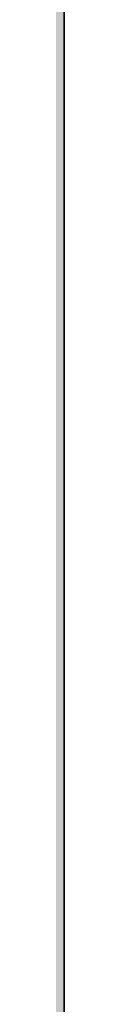
# Model space of a CAD drawing. Units: inches. Extents: x 2083 to 3317, y 1141 to 2115.
# Tile 214 of 256: x 3126.96 to 3126.96, y 1264.131 to 1265.165. Entities that reach past the tile are written whole.
import ezdxf

# ---------------------------------------------------------------- set-up
doc = ezdxf.new("R2010")
doc.units = ezdxf.units.IN
doc.layers.add('A-ANNO-DIMS', color=2, linetype='Continuous', lineweight=18)
doc.layers.add('A-WALL', color=7, linetype='Continuous', lineweight=35)
doc.layers.add('A-WALL-PATT', color=251, linetype='Continuous', lineweight=13, true_color=0x636466)
doc.styles.get("Standard").update_dxf_attribs({"font": 'arial.ttf'})
doc.dimstyles.new('ISO-25', dxfattribs={"dimtxt": 12, "dimasz": 12, "dimexe": 1.25, "dimexo": 0.625, "dimtad": 1, "dimlunit": 3, "dimtxsty": 'Standard', "dimcen": 2.5, "dimadec": 0, "dimazin": 0, "dimtfac": 1, "dimtmove": 0, "dimatfit": 3, "dimfxl": 1, "dimarcsym": 0})

# ---------------------------------------------------------------- blocks, each defined once
blk = doc.blocks.new('*D9')
at = {"layer": 'A-ANNO-DIMS', "color": 0, "lineweight": -2, "transparency": 16777216}
for p, q in [((3127.5848, 1486.7614), (3190.4031, 1486.7614)), ((3189.1531, 1474.7614), (3189.1531, 1275.2614)), ((3127.5848, 1263.2614), (3190.4031, 1263.2614))]:
    blk.add_line(p, q, dxfattribs=at)
at = {"layer": 'A-ANNO-DIMS', "color": 0, "transparency": 16777216}
for points in [[(3187.1531, 1474.7614), (3191.1531, 1474.7614), (3189.1531, 1486.7614)], [(3187.1531, 1275.2614), (3191.1531, 1275.2614), (3189.1531, 1263.2614)]]:
    blk.add_solid(points, dxfattribs=at)
at = {"layer": 'Defpoints', "color": 0, "transparency": 16777216}
for p in [(3126.9598, 1486.7614), (3126.9598, 1263.2614), (3189.1531, 1263.2614)]:
    blk.add_point(p, dxfattribs=at)
at = {"layer": 'A-ANNO-DIMS', "color": 0, "transparency": 16777216, "insert": (3182.4012, 1375.0114), "char_height": 12, "attachment_point": 5, "rotation": 90}
blk.add_mtext('18\'-7.5"', dxfattribs=at)
blk = doc.blocks.new('*D26')
at = {"layer": 'A-ANNO-DIMS', "color": 0, "lineweight": -2, "transparency": 16777216}
for p, q in [((3088.9858, 1274.9151), (3088.9858, 1270.952)), ((3111.24, 1274.9151), (3111.24, 1270.952)), ((3076.9858, 1272.202), (2840.2624, 1272.202)), ((3111.24, 1272.202), (3088.9858, 1272.202)), ((3123.24, 1272.202), (3135.24, 1272.202))]:
    blk.add_line(p, q, dxfattribs=at)
at = {"layer": 'A-ANNO-DIMS', "color": 0, "transparency": 16777216}
for points in [[(3076.9858, 1274.202), (3076.9858, 1270.202), (3088.9858, 1272.202)], [(3123.24, 1274.202), (3123.24, 1270.202), (3111.24, 1272.202)]]:
    blk.add_solid(points, dxfattribs=at)
at = {"layer": 'Defpoints', "color": 0, "transparency": 16777216}
for p in [(3088.9858, 1275.5401), (3111.24, 1275.5401), (3088.9858, 1272.202)]:
    blk.add_point(p, dxfattribs=at)
at = {"layer": 'A-ANNO-DIMS', "color": 0, "transparency": 16777216, "insert": (2952.6241, 1279.0316), "char_height": 12, "attachment_point": 5}
blk.add_mtext('NIGHTSTAND 1\'-10 1/2" TYP.', dxfattribs=at)
blk = doc.blocks.new('*D27')
at = {"layer": 'A-ANNO-DIMS', "color": 0, "lineweight": -2, "transparency": 16777216}
for p, q in [((3114.5782, 1309.7943), (3114.5782, 1321.7943)), ((3111.865, 1297.7943), (3115.8282, 1297.7943)), ((3114.5782, 1297.7943), (3114.5782, 1275.5401)), ((3111.865, 1275.5401), (3115.8282, 1275.5401)), ((3114.5782, 1263.5401), (3114.5782, 1140.9886))]:
    blk.add_line(p, q, dxfattribs=at)
at = {"layer": 'A-ANNO-DIMS', "color": 0, "transparency": 16777216}
for points in [[(3112.5782, 1309.7943), (3116.5782, 1309.7943), (3114.5782, 1297.7943)], [(3112.5782, 1263.5401), (3116.5782, 1263.5401), (3114.5782, 1275.5401)]]:
    blk.add_solid(points, dxfattribs=at)
at = {"layer": 'Defpoints', "color": 0, "transparency": 16777216}
for p in [(3111.24, 1297.7943), (3111.24, 1275.5401), (3114.5782, 1275.5401)]:
    blk.add_point(p, dxfattribs=at)
at = {"layer": 'A-ANNO-DIMS', "color": 0, "transparency": 16777216, "insert": (3107.7485, 1196.2643), "char_height": 12, "attachment_point": 5, "rotation": 90}
blk.add_mtext('1\'-10 1/2" TYP.', dxfattribs=at)

msp = doc.modelspace()

# ---------------------------------------------------------------- hatches: boundary and pattern name
at = {"layer": 'A-WALL-PATT'}
h = msp.add_hatch(color=256, dxfattribs=at)
h.dxf.hatch_style = 1
h.paths.add_polyline_path([(3126.9598, 2020.7614), (2748.9598, 2020.7614), (2604.9598, 2020.7614), (2226.9598, 2020.7614), (2226.9598, 1702.7614), (2466.9598, 1702.7614), (2466.9598, 1582.7614), (2418.9598, 1582.7614), (2418.9598, 1477.7614), (2226.9598, 1477.7614), (2226.9598, 1263.2614), (2544.9598, 1263.2614), (2544.9598, 1411.7614), (2604.9598, 1411.7614), (2685.9598, 1411.7614), (2685.9598, 1420.7614), (2604.9598, 1420.7614), (2604.9598, 1573.7614), (2604.9598, 1702.7614), (2604.9598, 2011.7614), (2748.9598, 2011.7614), (2748.9598, 1702.7614), (2862.9598, 1702.7614), (2862.9598, 1621.7614), (2871.9598, 1621.7614), (2871.9598, 1702.7614), (2883.9598, 1702.7614), (2883.9598, 1706.9395, -0.026459), (2883.9598, 1711.7614), (2757.9598, 1711.7614), (2757.9598, 1807.7614), (2787.9598, 1807.7614), (2787.9598, 1812.2614), (2757.9598, 1812.2614), (2757.9598, 2011.7614), (2877.9598, 2011.7614), (2877.9598, 1812.2614), (2847.9598, 1812.2614), (2847.9598, 1807.7614), (2889.8357, 1807.7614), (2889.8357, 1812.2614), (2882.4598, 1812.2614), (2882.4598, 2011.7614), (3117.9598, 2011.7614), (3117.9598, 1812.2614), (2937.8357, 1812.2614), (2937.8357, 1807.7614), (2995.7098, 1807.7614), (2995.7098, 1796.1177), (3000.2098, 1796.1177), (3000.2098, 1807.7614), (3117.9598, 1807.7614), (3117.9598, 1711.7614), (3000.2098, 1711.7614), (3000.2098, 1760.1177), (2998.5727, 1760.1177, -0.020711), (2995.7098, 1760.1177), (2995.7098, 1711.7614), (2931.9598, 1711.7614), (2931.9598, 1702.7614), (3126.9598, 1702.7614)])
h.paths.add_polyline_path([(2471.4598, 2011.7614), (2471.4598, 1810.0114), (2462.7169, 1810.0114), (2462.7169, 1805.5114), (2505.9598, 1805.5114), (2505.9598, 1810.0114), (2475.9598, 1810.0114), (2475.9598, 2011.7614), (2595.9598, 2011.7614), (2595.9598, 1810.0114), (2565.9598, 1810.0114), (2565.9598, 1805.5114), (2595.9598, 1805.5114), (2595.9598, 1711.7614), (2235.9598, 1711.7614), (2235.9598, 1805.5114), (2353.7098, 1805.5114), (2353.7098, 1796.0542), (2358.2098, 1796.0542), (2358.2098, 1805.5114), (2414.7169, 1805.5114), (2414.7169, 1810.0114), (2235.9598, 1810.0114), (2235.9598, 2011.7614)], flags=16)
h.paths.add_polyline_path([(2270.2047, 1994.61), (2270.2047, 1970.61), (2246.2047, 1970.61), (2246.2047, 1994.61)], flags=0)
edge = h.paths.add_edge_path(flags=0)
edge.add_ellipse((2332.0274, 1899.7982), major_axis=(-3.043, 3.043), ratio=0.168252, start_angle=-161.3322, end_angle=-156.3071, ccw=False)
edge.add_ellipse((2333.082, 1898.7435), major_axis=(-1.0546, 1.0546), ratio=0.453532, start_angle=-123.371, end_angle=-94.1591)
edge = h.paths.add_edge_path(flags=0)
edge.add_ellipse((2332.0274, 1968.8763), major_axis=(3.043, 3.043), ratio=0.168252, start_angle=18.6678, end_angle=23.6929)
edge.add_spline(control_points=[(2332.9256, 1970.6911), (2332.2268, 1970.3361), (2330.8937, 1969.6589), (2328.4131, 1970.9321), (2327.2039, 1967.7487), (2324.7096, 1969.9556), (2322.5328, 1967.0124), (2320.0128, 1971.2958), (2317.6803, 1968.1578), (2316.0405, 1967.102), (2315.4269, 1966.8096)], knot_values=[0, 0, 0, 0, 2.267059, 4.324559, 6.685584, 8.878641, 11.121502, 14.300359, 17.755284, 19.732645, 19.732645, 19.732645, 19.732645], degree=3, periodic=0)
edge.add_ellipse((2332.0274, 1968.8763), major_axis=(3.043, 3.043), ratio=0.168252, start_angle=18.6678, end_angle=23.6929, ccw=False)
edge.add_ellipse((2333.082, 1969.9309), major_axis=(1.0546, 1.0546), ratio=0.453532, start_angle=56.629, end_angle=85.8409, ccw=False)
edge = h.paths.add_edge_path(flags=0)
edge.add_spline(control_points=[(2296.4283, 1967.9879), (2293.6278, 1965.3363), (2287.7036, 1959.7271), (2299.7439, 1949.9957), (2294.5326, 1935.6685), (2290.5732, 1920.6035), (2293.3941, 1909.9737), (2296.1854, 1904.9665)], knot_values=[0.099185, 0.099185, 0.099185, 0.099185, 0.345301, 0.619822, 0.982653, 1.386093, 1.810555, 1.810555, 1.810555, 1.810555], degree=3, periodic=0)
edge.add_spline(control_points=[(2296.1854, 1904.9665), (2297.3836, 1902.6193), (2298.001, 1901.9493), (2298.553, 1901.4682)], knot_values=[0.006246, 0.006246, 0.006246, 0.006246, 0.055476, 0.055476, 0.055476, 0.055476], degree=3, periodic=0)
edge.add_spline(control_points=[(2298.553, 1901.4682), (2297.2586, 1900.9232), (2295.2253, 1900.2321), (2293.0602, 1900.6142), (2292.1014, 1900.7884), (2292.0896, 1900.7906)], knot_values=[0.312835, 0.312835, 0.312835, 0.312835, 0.40178, 0.474987, 0.475903, 0.475903, 0.475903, 0.475903], degree=3, periodic=0)
edge.add_arc((2292.7936, 1904.6641), 3.937, 215.4209, 259.6982, ccw=False)
edge.add_spline(control_points=[(2289.5853, 1902.3823), (2289.4767, 1902.5351), (2289.3685, 1902.688), (2289.2609, 1902.8412)], knot_values=[0.102872, 0.102872, 0.102872, 0.102872, 0.116896, 0.116896, 0.116896, 0.116896], degree=3, periodic=0)
edge.add_spline(control_points=[(2289.2609, 1902.8412), (2288.6866, 1902.5502), (2287.64, 1902.0199), (2285.8813, 1901.874), (2283.853, 1901.5044), (2281.72, 1899.7105), (2278.467, 1899.4929), (2276.1571, 1901.8832), (2272.259, 1899.8041), (2267.7776, 1901.8432), (2262.2439, 1900.184), (2257.4149, 1901.7821), (2254.3184, 1900.7261), (2253.1783, 1900.3373)], knot_values=[0, 0, 0, 0, 1.907977, 3.477176, 5.261074, 7.972851, 11.680248, 13.717921, 16.939592, 22.789562, 27.502503, 33.595215, 37.145618, 37.145618, 37.145618, 37.145618], degree=3, periodic=0)
edge.add_line((2253.1783, 1900.3373), (2250.2442, 1902.8412))
edge.add_line((2250.2442, 1902.8412), (2250.2442, 1965.8333))
edge.add_line((2250.2442, 1965.8333), (2253.1783, 1968.3371))
edge.add_spline(control_points=[(2253.1783, 1968.3371), (2254.3184, 1967.9483), (2257.4149, 1966.8924), (2262.2439, 1968.4904), (2267.7776, 1966.8313), (2271.5267, 1968.5372), (2273.8759, 1967.8283), (2274.2067, 1967.7276)], knot_values=[0, 0, 0, 0, 0.09018, 0.244935, 0.364644, 0.513233, 0.537855, 0.537855, 0.537855, 0.537855], degree=3, periodic=0)
edge.add_arc((2274.3529, 1963.7933), 3.937, 72.0511, 92.1279, ccw=False)
edge.add_arc((2281.2969, 1985.23), 18.5963, 252.05113, 288.56572)
edge.add_arc((2292.3167, 1956.0289), 12.6461, 71.02679, 113.77822, ccw=False)
edge = h.paths.add_edge_path(flags=0)
edge.add_spline(control_points=[(2274.8994, 1951.8562), (2275.0662, 1951.6166), (2275.2327, 1951.3766), (2275.398, 1951.1359)], knot_values=[1.409916, 1.409916, 1.409916, 1.409916, 1.43159, 1.43159, 1.43159, 1.43159], degree=3, periodic=0)
edge.add_spline(control_points=[(2275.398, 1951.1359), (2275.7921, 1950.5619), (2276.1792, 1949.9838), (2276.5455, 1949.3971)], knot_values=[1.358238, 1.358238, 1.358238, 1.358238, 1.409916, 1.409916, 1.409916, 1.409916], degree=3, periodic=0)
edge.add_line((2276.5455, 1949.3971), (2277.4373, 1947.8622))
edge.add_spline(control_points=[(2277.4373, 1947.8622), (2276.3038, 1945.6731), (2274.6397, 1942.4269), (2274.6316, 1938.0939), (2272.7991, 1930.8515), (2274.3564, 1943.897), (2275.9477, 1947.9234), (2276.5455, 1949.3971)], knot_values=[0.005632, 0.005632, 0.005632, 0.005632, 0.186014, 0.266002, 0.357087, 0.59639, 0.739732, 0.739732, 0.739732, 0.739732], degree=3, periodic=0)
edge.add_spline(control_points=[(2276.5455, 1949.3971), (2276.1792, 1949.9838), (2275.7921, 1950.5619), (2275.398, 1951.1359)], knot_values=[1.358238, 1.358238, 1.358238, 1.358238, 1.409916, 1.409916, 1.409916, 1.409916], degree=3, periodic=0)
edge.add_spline(control_points=[(2275.398, 1951.1359), (2274.9425, 1950.0805), (2274.2078, 1948.0253), (2273.9346, 1944.8515), (2272.4685, 1937.6275), (2273.4662, 1945.6965), (2274.7006, 1951.0595), (2274.8994, 1951.8562)], knot_values=[0.104364, 0.104364, 0.104364, 0.104364, 0.189636, 0.269624, 0.36071, 0.600013, 0.644622, 0.644622, 0.644622, 0.644622], degree=3, periodic=0)
h.paths.add_polyline_path([(2269.1675, 1963.1276, -0.357527), (2268.1706, 1960.9764, -0.092561), (2268.1706, 1939.4363, -0.357527), (2269.1675, 1937.2851, -0.357527), (2267.0163, 1938.282, -0.164785), (2254.6856, 1938.282, -0.357527), (2252.5344, 1937.2851, -0.357527), (2253.5313, 1939.4363, -0.092561), (2253.5313, 1960.9764, -0.357527), (2252.5344, 1963.1276, -0.357527), (2254.6856, 1962.1307, -0.164785), (2267.0163, 1962.1307, -0.357527)], flags=0)
h.paths.add_polyline_path([(2248.8741, 1967.8018), (2248.8741, 1957.0277), (2249.4578, 1957.0277), (2249.4578, 1911.6468), (2248.8741, 1911.6468), (2248.8741, 1900.8727), (2246.5119, 1900.8727, 0.197327), (2244.1497, 1902.4569), (2244.1497, 1966.2176, 0.197327), (2246.5119, 1967.8018)], flags=0)
h.paths.add_polyline_path([(2269.1675, 1931.3893, -0.357527), (2268.1706, 1929.2381, -0.092561), (2268.1706, 1907.6981, -0.357527), (2269.1675, 1905.5469, -0.357527), (2267.0163, 1906.5438, -0.164785), (2254.6856, 1906.5438, -0.357527), (2252.5344, 1905.5469, -0.357527), (2253.5313, 1907.6981, -0.092561), (2253.5313, 1929.2381, -0.357527), (2252.5344, 1931.3893, -0.357527), (2254.6856, 1930.3925, -0.164785), (2267.0163, 1930.3925, -0.357527)], flags=0)
edge = h.paths.add_edge_path(flags=0)
edge.add_spline(control_points=[(2276.1969, 1906.7237), (2276.1681, 1909.0289), (2276.114, 1913.3719), (2270.5984, 1924.925), (2273.9052, 1919.0128), (2275.9217, 1916.2621), (2275.4746, 1912.4021), (2277.2579, 1910.3806), (2276.696, 1908.225), (2276.6462, 1906.813), (2276.6178, 1906.0084)], knot_values=[0, 0, 0, 0, 8.61026, 16.221274, 18.843057, 23.804898, 27.440828, 29.356102, 31.203478, 33.650687, 33.650687, 33.650687, 33.650687], degree=3, periodic=0)
edge.add_spline(control_points=[(2276.6178, 1906.0084), (2276.6233, 1905.6241), (2276.4977, 1904.6287), (2275.4418, 1903.8547), (2274.9373, 1903.0804), (2274.8591, 1902.8412)], knot_values=[0.156488, 0.156488, 0.156488, 0.156488, 0.184398, 0.231376, 0.250598, 0.250598, 0.250598, 0.250598], degree=3, periodic=0)
edge.add_line((2274.8591, 1902.8412), (2276.506, 1902.8412))
edge.add_spline(control_points=[(2276.506, 1902.8412), (2276.7883, 1903.0849), (2277.6651, 1904.1252), (2278.2495, 1904.3407), (2277.6539, 1908.5274), (2278.1557, 1906.2278), (2278.1005, 1905.2859), (2278.8467, 1904.069), (2277.8568, 1903.4149), (2277.8742, 1902.991), (2277.9036, 1902.8412)], knot_values=[0.059574, 0.059574, 0.059574, 0.059574, 0.080753, 0.103741, 0.16972, 0.176036, 0.207137, 0.240474, 0.262341, 0.27366, 0.27366, 0.27366, 0.27366], degree=3, periodic=0)
edge.add_line((2277.9036, 1902.8412), (2280.0298, 1902.8412))
edge.add_spline(control_points=[(2280.0298, 1902.8412), (2279.8882, 1903.0884), (2279.4993, 1903.9816), (2280.1523, 1905.9393), (2278.1036, 1909.6578), (2279.7624, 1907.1853), (2280.3279, 1904.8749), (2280.4851, 1903.4896), (2281.4633, 1903.2494), (2281.7583, 1902.9365), (2281.834, 1902.8412)], knot_values=[0.013856, 0.013856, 0.013856, 0.013856, 0.034874, 0.088867, 0.107879, 0.126738, 0.158714, 0.193757, 0.217487, 0.226722, 0.226722, 0.226722, 0.226722], degree=3, periodic=0)
edge.add_spline(control_points=[(2281.834, 1902.8412), (2281.7875, 1902.8267), (2281.647, 1902.783), (2281.3955, 1902.8595), (2281.0881, 1902.9852), (2280.7207, 1903.0609), (2280.3335, 1903.0257), (2280.1248, 1902.8989), (2280.0298, 1902.8412)], knot_values=[0, 0, 0, 0, 0.14413, 0.435517, 0.749276, 1.153046, 1.548371, 1.878348, 1.878348, 1.878348, 1.878348], degree=3, periodic=0)
edge.add_line((2280.0298, 1902.8412), (2277.9036, 1902.8412))
edge.add_spline(control_points=[(2277.9036, 1902.8412), (2277.8929, 1902.7959), (2277.8654, 1902.6796), (2277.6075, 1902.6875), (2277.2741, 1902.8007), (2276.8379, 1902.6198), (2276.5838, 1902.7893), (2276.506, 1902.8412)], knot_values=[0, 0, 0, 0, 0.127189, 0.326199, 0.628009, 1.24357, 1.515331, 1.515331, 1.515331, 1.515331], degree=3, periodic=0)
edge.add_line((2276.506, 1902.8412), (2274.8591, 1902.8412))
edge.add_spline(control_points=[(2274.8591, 1902.8412), (2274.8144, 1902.8986), (2274.7251, 1903.0134), (2274.4935, 1903.119), (2274.2443, 1902.9605), (2273.9371, 1903.1849), (2273.614, 1902.9831), (2273.4083, 1902.883), (2273.3223, 1902.8412)], knot_values=[0, 0, 0, 0, 0.21843, 0.436957, 0.687977, 0.990379, 1.398396, 1.69185, 1.69185, 1.69185, 1.69185], degree=3, periodic=0)
edge.add_spline(control_points=[(2273.3223, 1902.8412), (2273.6167, 1903.4457), (2274.274, 1904.5383), (2276.0272, 1904.5737), (2276.207, 1906.5836), (2276.1969, 1906.7237)], knot_values=[0.012227, 0.012227, 0.012227, 0.012227, 0.059472, 0.106218, 0.134458, 0.134458, 0.134458, 0.134458], degree=3, periodic=0)
h.paths.add_polyline_path([(2270.7761, 1897.7898), (2270.7761, 1873.7898), (2246.7761, 1873.7898), (2246.7761, 1897.7898)], flags=0)
h.paths.add_polyline_path([(2353.7098, 1760.0051), (2353.7098, 1760.0542), (2358.2098, 1760.0542, -0.033729)], flags=0)
h.paths.add_polyline_path([(2321.8191, 1737.5292), (2341.9953, 1737.5292, -0.414214), (2343.2033, 1736.3212), (2343.2033, 1721.0206, -0.414214), (2341.9953, 1719.8127), (2321.8191, 1719.8127, -0.414214), (2320.6112, 1721.0206), (2320.6112, 1736.3212, -0.414214)], flags=0)
h.paths.add_polyline_path([(2324.235, 1736.3212), (2339.5794, 1736.3212, -0.414214), (2341.9953, 1733.9053), (2341.9953, 1725.4497, -0.414214), (2339.5794, 1723.0338), (2333.6806, 1723.0338), (2333.8453, 1722.0455, -0.870646), (2335.4254, 1721.8259, -0.767327), (2333.9227, 1721.4232), (2331.291, 1721.4232, -0.767327), (2329.7883, 1721.8259, -0.870646), (2331.3684, 1722.0455), (2331.5331, 1723.0338), (2324.235, 1723.0338, -0.414214), (2321.8191, 1725.4497), (2321.8191, 1733.9053, -0.414214)], flags=0)
h.paths.add_polyline_path([(2570.4838, 1928.6154), (2589.6838, 1928.6154), (2590.1688, 1928.6154), (2590.1688, 1904.9934), (2570.4838, 1904.9934)], flags=0)
h.paths.add_polyline_path([(2574.4473, 1927.2638, -1), (2572.8288, 1927.2638, -1)], flags=0)
h.paths.add_polyline_path([(2573.0899, 1926.9409), (2573.925, 1927.776), (2574.1477, 1927.5533), (2573.3126, 1926.7182)], flags=0)
h.paths.add_polyline_path([(2578.7791, 1919.7296, -1), (2571.5917, 1919.7296, -1)], flags=0)
h.paths.add_polyline_path([(2578.3854, 1919.7296, -1), (2571.9854, 1919.7296, -1)], flags=0)
h.paths.add_polyline_path([(2331.5958, 1729.4762, -1), (2333.618, 1729.4762, -1)], flags=0)
h.paths.add_polyline_path([(2578.0342, 1927.2638, -1), (2576.4157, 1927.2638, -1)], flags=0)
h.paths.add_polyline_path([(2576.6889, 1927.5311), (2576.9116, 1927.7538), (2577.7467, 1926.9186), (2577.524, 1926.6959)], flags=0)
h.paths.add_polyline_path([(2578.1391, 1909.8595, -1), (2572.2317, 1909.8595, -1)], flags=0)
h.paths.add_polyline_path([(2577.7454, 1909.8595, -1), (2572.6254, 1909.8595, -1)], flags=0)
h.paths.add_polyline_path([(2583.7977, 1927.2638, -1), (2582.1792, 1927.2638, -1)], flags=0)
h.paths.add_polyline_path([(2582.7186, 1927.7538), (2583.5538, 1926.9186), (2583.3311, 1926.6959), (2582.4959, 1927.5311)], flags=0)
h.paths.add_polyline_path([(2582.4959, 1927.5311), (2582.7186, 1927.7538), (2583.5538, 1926.9186), (2583.3311, 1926.6959)], flags=0)
h.paths.add_polyline_path([(2587.7391, 1920.5296, -1), (2581.8317, 1920.5296, -1)], flags=0)
h.paths.add_polyline_path([(2587.3454, 1920.5296, -1), (2582.2254, 1920.5296, -1)], flags=0)
h.paths.add_polyline_path([(2587.3846, 1927.2638, -1), (2585.7661, 1927.2638, -1)], flags=0)
h.paths.add_polyline_path([(2586.082, 1926.9802), (2586.9172, 1927.8154), (2587.1399, 1927.5927), (2586.3047, 1926.7575)], flags=0)
h.paths.add_polyline_path([(2588.3791, 1910.6595, -1), (2581.1917, 1910.6595, -1)], flags=0)
h.paths.add_polyline_path([(2587.9854, 1910.6595, -1), (2581.5854, 1910.6595, -1)], flags=0)
h.paths.add_polyline_path([(2417.1677, 1729.4779), (2437.3439, 1729.4779, -0.414214), (2438.5519, 1728.2699), (2438.5519, 1712.9693, -0.414214), (2437.3439, 1711.7614), (2417.1677, 1711.7614, -0.414214), (2415.9598, 1712.9693), (2415.9598, 1728.2699, -0.414214)], flags=0)
h.paths.add_polyline_path([(2419.5836, 1728.2699), (2434.928, 1728.2699, -0.414214), (2437.3439, 1725.8541), (2437.3439, 1717.3984, -0.414214), (2434.928, 1714.9825), (2429.0292, 1714.9825), (2429.1939, 1713.9942, -0.870646), (2430.774, 1713.7746, -0.767327), (2429.2713, 1713.372), (2426.6396, 1713.372, -0.767327), (2425.1369, 1713.7746, -0.870646), (2426.717, 1713.9942), (2426.8817, 1714.9825), (2419.5836, 1714.9825, -0.414214), (2417.1677, 1717.3984), (2417.1677, 1725.8541, -0.414214)], flags=0)
h.paths.add_polyline_path([(2419.5836, 1728.2699), (2434.928, 1728.2699, -0.414214), (2437.3439, 1725.8541), (2437.3439, 1717.3984, -0.414214), (2434.928, 1714.9825), (2429.0292, 1714.9825), (2428.3581, 1719.009), (2427.5528, 1719.009), (2426.8817, 1714.9825), (2419.5836, 1714.9825, -0.414214), (2417.1677, 1717.3984), (2417.1677, 1725.8541, -0.414214)], flags=0)
h.paths.add_polyline_path([(2426.9444, 1721.4249, -1), (2428.9666, 1721.4249, -1)], flags=0)
h.paths.add_polyline_path([(2475.9598, 1702.7614), (2595.9598, 1702.7614), (2595.9598, 1582.7614), (2475.9598, 1582.7614)], flags=16)
h.paths.add_polyline_path([(2427.9598, 1573.7614), (2595.9598, 1573.7614), (2595.9598, 1468.7614), (2595.9598, 1420.7614), (2384.4598, 1420.7614), (2384.4598, 1468.7614), (2427.9598, 1468.7614)], flags=16)
h.paths.add_polyline_path([(2379.9598, 1468.7614), (2379.9598, 1420.7614), (2235.9598, 1420.7614), (2235.9598, 1468.7614)], flags=16)
h.paths.add_polyline_path([(2317.816, 1466.6958), (2337.9922, 1466.6958, -0.414214), (2339.2002, 1465.4878), (2339.2002, 1450.1872, -0.414214), (2337.9922, 1448.9792), (2317.816, 1448.9792, -0.414214), (2316.6081, 1450.1872), (2316.6081, 1465.4878, -0.414214)], flags=0)
h.paths.add_polyline_path([(2320.2319, 1465.4878), (2335.5763, 1465.4878, -0.414214), (2337.9922, 1463.0719), (2337.9922, 1454.6163, -0.414214), (2335.5763, 1452.2004), (2329.6775, 1452.2004), (2329.8422, 1451.212, -0.870646), (2331.4223, 1450.9925, -0.767327), (2329.9196, 1450.5898), (2327.2879, 1450.5898, -0.767327), (2325.7852, 1450.9925, -0.870646), (2327.3653, 1451.212), (2327.53, 1452.2004), (2320.2319, 1452.2004, -0.414214), (2317.816, 1454.6163), (2317.816, 1463.0719, -0.414214)], flags=0)
h.paths.add_polyline_path([(2320.2319, 1465.4878), (2335.5763, 1465.4878, -0.414214), (2337.9922, 1463.0719), (2337.9922, 1454.6163, -0.414214), (2335.5763, 1452.2004), (2329.6775, 1452.2004), (2329.0064, 1456.2269), (2328.2011, 1456.2269), (2327.53, 1452.2004), (2320.2319, 1452.2004, -0.414214), (2317.816, 1454.6163), (2317.816, 1463.0719, -0.414214)], flags=0)
h.paths.add_polyline_path([(2327.5926, 1458.6428, -1), (2329.6148, 1458.6428, -1)], flags=0)
h.paths.add_polyline_path([(2244.4117, 1433.3405), (2241.9209, 1433.3405, -0.414214), (2240.0179, 1435.2435), (2240.0179, 1440.9528, -0.414211), (2241.9209, 1442.8559), (2244.4117, 1442.8559, -1.976472)], flags=0)
h.paths.add_polyline_path([(2245.3569, 1434.3975, -0.414214), (2245.3569, 1441.7988, -2.144098)], flags=0)
h.paths.add_polyline_path([(2535.9598, 1416.2614), (2535.9598, 1272.2614), (2235.9598, 1272.2614), (2235.9598, 1416.2614)], flags=16)
h.paths.add_polyline_path([(2260.1196, 1384.2928), (2260.1196, 1362.0386), (2237.8654, 1362.0386), (2237.8654, 1384.2928)], flags=0)
edge = h.paths.add_edge_path(flags=0)
edge.add_line((2318.2518, 1362.0933), (2318.1458, 1362.001))
edge.add_ellipse((2317.4451, 1360.431), major_axis=(2.8216, 2.8216), ratio=0.168252, start_angle=18.6678, end_angle=20.9481, ccw=False)
edge.add_ellipse((2318.423, 1361.409), major_axis=(0.9779, 0.9779), ratio=0.453532, start_angle=56.629, end_angle=70.2262, ccw=False)
edge = h.paths.add_edge_path(flags=0)
edge.add_line((2319.1074, 1295.5711), (2319.015, 1295.6771))
edge.add_ellipse((2317.4451, 1296.3778), major_axis=(-2.8216, 2.8216), ratio=0.168252, start_angle=-161.3322, end_angle=-159.0519, ccw=False)
edge.add_ellipse((2318.423, 1295.3999), major_axis=(-0.9779, 0.9779), ratio=0.453532, start_angle=-123.371, end_angle=-109.7738)
edge = h.paths.add_edge_path(flags=0)
edge.add_spline(control_points=[(2284.2103, 1301.1702), (2284.5807, 1300.4447), (2284.8912, 1299.892), (2285.1596, 1299.461)], knot_values=[0.039066, 0.039066, 0.039066, 0.039066, 0.055476, 0.055476, 0.055476, 0.055476], degree=3, periodic=0)
edge.add_line((2285.1596, 1299.461), (2284.2103, 1301.1702))
edge = h.paths.add_edge_path(flags=0)
edge.add_line((2280.4125, 1297.298), (2283.37, 1297.0361))
edge.add_line((2283.37, 1297.0361), (2286.4057, 1297.9263))
edge.add_spline(control_points=[(2286.4057, 1297.9263), (2285.3055, 1297.4631), (2284.3448, 1297.1292), (2283.37, 1297.0361)], knot_values=[0.394369, 0.394369, 0.394369, 0.394369, 0.475903, 0.475903, 0.475903, 0.475903], degree=3, periodic=0)
edge.add_spline(control_points=[(2283.37, 1297.0361), (2283.2814, 1297.0277), (2282.3163, 1296.9573), (2281.3125, 1297.1345), (2280.4234, 1297.296), (2280.4125, 1297.298)], knot_values=[0.312835, 0.312835, 0.312835, 0.312835, 0.320246, 0.393453, 0.394369, 0.394369, 0.394369, 0.394369], degree=3, periodic=0)
edge = h.paths.add_edge_path(flags=0)
edge.add_line((2284.4356, 1359.6073), (2280.4463, 1355.328))
edge.add_line((2280.4463, 1355.328), (2279.58, 1351.0178))
edge.add_line((2279.58, 1351.0178), (2282.413, 1346.5804))
edge.add_spline(control_points=[(2282.413, 1346.5804), (2283.1533, 1345.5892), (2284.2529, 1344.0289), (2284.801, 1342.3872), (2284.9352, 1341.8055)], knot_values=[1.240098, 1.240098, 1.240098, 1.240098, 1.332892, 1.382712, 1.382712, 1.382712, 1.382712], degree=3, periodic=0)
edge.add_spline(control_points=[(2284.9352, 1341.8055), (2285.3191, 1340.1406), (2285.233, 1338.4092), (2284.9099, 1336.6541)], knot_values=[1.097484, 1.097484, 1.097484, 1.097484, 1.240098, 1.240098, 1.240098, 1.240098], degree=3, periodic=0)
edge.add_spline(control_points=[(2284.9099, 1336.6541), (2284.5868, 1334.899), (2284.0267, 1333.1203), (2283.4626, 1331.3606)], knot_values=[0.95487, 0.95487, 0.95487, 0.95487, 1.097484, 1.097484, 1.097484, 1.097484], degree=3, periodic=0)
edge.add_line((2283.4626, 1331.3606), (2281.8904, 1326.1534))
edge.add_line((2281.8904, 1326.1534), (2280.7563, 1321.0561))
edge.add_line((2280.7563, 1321.0561), (2280.2992, 1316.002))
edge.add_line((2280.2992, 1316.002), (2280.7159, 1310.9501))
edge.add_line((2280.7159, 1310.9501), (2282.0281, 1305.9721))
edge.add_line((2282.0281, 1305.9721), (2284.2103, 1301.1702))
edge.add_spline(control_points=[(2284.2103, 1301.1702), (2283.3407, 1302.7302), (2282.6119, 1304.3365), (2282.0281, 1305.9721)], knot_values=[0.099185, 0.099185, 0.099185, 0.099185, 0.241799, 0.241799, 0.241799, 0.241799], degree=3, periodic=0)
edge.add_spline(control_points=[(2282.0281, 1305.9721), (2281.4443, 1307.6078), (2281.0055, 1309.2728), (2280.7159, 1310.9501)], knot_values=[0.241799, 0.241799, 0.241799, 0.241799, 0.384413, 0.384413, 0.384413, 0.384413], degree=3, periodic=0)
edge.add_spline(control_points=[(2280.7159, 1310.9501), (2280.4332, 1312.5876), (2280.2894, 1314.277), (2280.2989, 1315.962), (2280.2992, 1316.002)], knot_values=[0.384413, 0.384413, 0.384413, 0.384413, 0.523647, 0.527028, 0.527028, 0.527028, 0.527028], degree=3, periodic=0)
edge.add_spline(control_points=[(2280.2992, 1316.002), (2280.3123, 1317.687), (2280.4779, 1319.3679), (2280.7563, 1321.0561)], knot_values=[0.527028, 0.527028, 0.527028, 0.527028, 0.669642, 0.669642, 0.669642, 0.669642], degree=3, periodic=0)
edge.add_spline(control_points=[(2280.7563, 1321.0561), (2281.0346, 1322.7443), (2281.4259, 1324.4396), (2281.8904, 1326.1534)], knot_values=[0.669642, 0.669642, 0.669642, 0.669642, 0.812256, 0.812256, 0.812256, 0.812256], degree=3, periodic=0)
edge.add_spline(control_points=[(2281.8904, 1326.1534), (2282.2644, 1327.5333), (2282.7879, 1329.2618), (2283.3528, 1331.0178), (2283.4626, 1331.3606)], knot_values=[0.812256, 0.812256, 0.812256, 0.812256, 0.927087, 0.95487, 0.95487, 0.95487, 0.95487], degree=3, periodic=0)
edge.add_line((2283.4626, 1331.3606), (2284.9099, 1336.6541))
edge.add_line((2284.9099, 1336.6541), (2284.9352, 1341.8055))
edge.add_line((2284.9352, 1341.8055), (2282.413, 1346.5804))
edge.add_spline(control_points=[(2282.413, 1346.5804), (2281.2751, 1348.1038), (2280.0784, 1349.5703), (2279.58, 1351.0178)], knot_values=[1.382712, 1.382712, 1.382712, 1.382712, 1.525326, 1.525326, 1.525326, 1.525326], degree=3, periodic=0)
edge.add_spline(control_points=[(2279.58, 1351.0178), (2279.4433, 1351.4147), (2279.1363, 1352.8569), (2279.7352, 1354.2904), (2280.4463, 1355.328)], knot_values=[1.525326, 1.525326, 1.525326, 1.525326, 1.564439, 1.667941, 1.667941, 1.667941, 1.667941], degree=3, periodic=0)
edge.add_spline(control_points=[(2280.4463, 1355.328), (2281.4261, 1356.7578), (2282.9308, 1358.1826), (2284.4356, 1359.6073)], knot_values=[1.667941, 1.667941, 1.667941, 1.667941, 1.810555, 1.810555, 1.810555, 1.810555], degree=3, periodic=0)
edge.add_arc((2280.6231, 1348.5182), 11.7262, 71.02679, 113.77822)
edge.add_arc((2270.4049, 1375.5952), 17.2436, 252.05113, 288.56572, ccw=False)
edge.add_arc((2263.966, 1355.7178), 3.6506, 72.0511, 92.1279)
edge.add_arc((2263.966, 1355.7178), 3.6506, 92.1279, 177.9851)
edge.add_spline(control_points=[(2260.3176, 1355.8462), (2260.2604, 1354.2207), (2260.5513, 1350.1865), (2262.9993, 1346.7663), (2264.4727, 1344.649)], knot_values=[1.43159, 1.43159, 1.43159, 1.43159, 1.564144, 1.770695, 1.770695, 1.770695, 1.770695], degree=3, periodic=0)
edge.add_line((2264.4727, 1344.649), (2264.9356, 1343.9825))
edge.add_spline(control_points=[(2263.801, 1340.2481), (2263.8432, 1340.5141), (2264.0672, 1341.7565), (2264.5127, 1343.0025), (2264.935, 1343.9811)], knot_values=[0.53657, 0.53657, 0.53657, 0.53657, 0.559349, 0.644622, 0.644622, 0.644622, 0.644622], degree=3, periodic=0)
edge.add_spline(control_points=[(2264.935, 1343.9811), (2265.1178, 1343.715), (2265.2989, 1343.4479), (2265.4768, 1343.1794)], knot_values=[1.384077, 1.384077, 1.384077, 1.384077, 1.409916, 1.409916, 1.409916, 1.409916], degree=3, periodic=0)
edge.add_spline(control_points=[(2265.4768, 1343.1794), (2265.6546, 1342.9108), (2265.8293, 1342.6408), (2265.9991, 1342.3688)], knot_values=[1.358238, 1.358238, 1.358238, 1.358238, 1.384077, 1.384077, 1.384077, 1.384077], degree=3, periodic=0)
edge.add_line((2265.9991, 1342.3688), (2266.826, 1340.9455))
edge.add_spline(control_points=[(2266.826, 1340.9455), (2268.8944, 1337.0897), (2271.3982, 1325.843), (2270.5162, 1310.5686), (2275.9194, 1301.8606), (2277.7895, 1299.1994)], knot_values=[0.116896, 0.116896, 0.116896, 0.116896, 0.472987, 1.050969, 1.313793, 1.313793, 1.313793, 1.313793], degree=3, periodic=0)
edge.add_spline(control_points=[(2277.7895, 1299.1994), (2277.8394, 1299.1285), (2277.8894, 1299.0575), (2277.9396, 1298.9866)], knot_values=[0.109884, 0.109884, 0.109884, 0.109884, 0.116896, 0.116896, 0.116896, 0.116896], degree=3, periodic=0)
edge.add_line((2277.9396, 1298.9866), (2277.7888, 1299.1991))
edge.add_spline(control_points=[(2277.7888, 1299.1991), (2277.2566, 1298.9294), (2276.2864, 1298.4379), (2275.0394, 1298.3344), (2274.3833, 1298.2389), (2274.2153, 1298.2093)], knot_values=[33.12187, 33.12187, 33.12187, 33.12187, 35.029056, 36.598255, 37.144827, 37.144827, 37.144827, 37.144827], degree=3, periodic=0)
edge.add_line((2274.2153, 1298.2093), (2273.0731, 1297.893))
edge.add_spline(control_points=[(2273.0731, 1297.893), (2272.3229, 1297.5798), (2271.0392, 1296.5105), (2269.2484, 1296.2261), (2268.4231, 1296.3747)], knot_values=[26.532584, 26.532584, 26.532584, 26.532584, 29.198919, 31.839101, 31.839101, 31.839101, 31.839101], degree=3, periodic=0)
edge.add_line((2268.4231, 1296.3747), (2263.8785, 1297.4575))
edge.add_spline(control_points=[(2263.8785, 1297.4575), (2263.5561, 1297.3594), (2261.8603, 1296.8387), (2260.2388, 1297.2824), (2258.9335, 1297.5165)], knot_values=[15.919551, 15.919551, 15.919551, 15.919551, 16.939592, 21.226067, 21.226067, 21.226067, 21.226067], degree=3, periodic=0)
edge.add_line((2258.9335, 1297.5165), (2254.0552, 1297.329))
edge.add_spline(control_points=[(2254.0552, 1297.329), (2253.7555, 1297.2958), (2252.1137, 1297.1652), (2250.4619, 1297.5442), (2249.1297, 1297.6679)], knot_values=[5.306517, 5.306517, 5.306517, 5.306517, 6.276435, 10.613034, 10.613034, 10.613034, 10.613034], degree=3, periodic=0)
edge.add_line((2249.1297, 1297.6679), (2244.3316, 1296.8778))
edge.add_line((2244.3316, 1296.8778), (2241.611, 1299.1994))
edge.add_line((2241.611, 1299.1994), (2241.611, 1357.6094))
edge.add_line((2241.611, 1357.6094), (2244.3316, 1359.9311))
edge.add_line((2244.3316, 1359.9311), (2252.7288, 1359.5427))
edge.add_spline(control_points=[(2252.7288, 1359.5427), (2252.8709, 1359.5464), (2253.3057, 1359.5482), (2253.7398, 1359.5143), (2254.0317, 1359.4824)], knot_values=[0.233291, 0.233291, 0.233291, 0.233291, 0.244935, 0.268927, 0.268927, 0.268927, 0.268927], degree=3, periodic=0)
edge.add_line((2254.0317, 1359.4824), (2259.5872, 1359.4164))
edge.add_spline(control_points=[(2259.5872, 1359.4164), (2260.6771, 1359.6285), (2262.0732, 1359.897), (2263.5237, 1359.4593), (2263.8304, 1359.366)], knot_values=[0.422516, 0.422516, 0.422516, 0.422516, 0.513233, 0.537855, 0.537855, 0.537855, 0.537855], degree=3, periodic=0)
edge.add_arc((2263.966, 1355.7178), 3.6506, 72.0511, 92.1279, ccw=False)
edge.add_arc((2270.4049, 1375.5952), 17.2436, 252.05113, 288.56572)
edge.add_arc((2280.6231, 1348.5182), 11.7262, 71.02679, 113.77822, ccw=False)
h.paths.add_polyline_path([(2240.3405, 1359.4347), (2240.3405, 1349.4444), (2240.8818, 1349.4444), (2240.8818, 1307.3645), (2240.3405, 1307.3645), (2240.3405, 1297.3741), (2238.1502, 1297.3741, 0.197327), (2235.9598, 1298.8431), (2235.9598, 1357.9657, 0.197327), (2238.1502, 1359.4347)], flags=0)
h.paths.add_polyline_path([(2259.1578, 1355.1005, -0.357527), (2258.2334, 1353.1058, -0.092561), (2258.2334, 1333.1326, -0.357527), (2259.1578, 1331.1379, -0.357527), (2257.1631, 1332.0622, -0.164785), (2245.7293, 1332.0622, -0.357527), (2243.7346, 1331.1379, -0.357527), (2244.6589, 1333.1326, -0.092561), (2244.6589, 1353.1058, -0.357527), (2243.7346, 1355.1005, -0.357527), (2245.7293, 1354.1761, -0.164785), (2257.1631, 1354.1761, -0.357527)], flags=0)
edge = h.paths.add_edge_path(flags=0)
edge.add_line((2265.9991, 1342.3688), (2266.826, 1340.9455))
edge.add_line((2266.826, 1340.9455), (2265.3076, 1337.8141))
edge.add_line((2265.3076, 1337.8141), (2264.3582, 1334.6529))
edge.add_line((2264.3582, 1334.6529), (2264.262, 1333.7997))
edge.add_spline(control_points=[(2264.262, 1333.7997), (2264.2084, 1333.1871), (2264.1621, 1332.3655), (2264.0071, 1331.4139), (2263.969, 1331.2018)], knot_values=[0.464444, 0.464444, 0.464444, 0.464444, 0.516691, 0.531608, 0.531608, 0.531608, 0.531608], degree=3, periodic=0)
edge.add_spline(control_points=[(2263.969, 1331.2018), (2263.7745, 1330.1189), (2263.4244, 1328.7908), (2263.2574, 1328.5307), (2263.234, 1328.5146)], knot_values=[0.372682, 0.372682, 0.372682, 0.372682, 0.44885, 0.464444, 0.464444, 0.464444, 0.464444], degree=3, periodic=0)
edge.add_spline(control_points=[(2263.234, 1328.5146), (2263.0964, 1328.4202), (2263.1312, 1329.3015), (2263.275, 1330.6157)], knot_values=[0.280919, 0.280919, 0.280919, 0.280919, 0.372682, 0.372682, 0.372682, 0.372682], degree=3, periodic=0)
edge.add_spline(control_points=[(2263.275, 1330.6157), (2263.4187, 1331.93), (2263.6715, 1333.6773), (2263.9699, 1335.315)], knot_values=[0.189157, 0.189157, 0.189157, 0.189157, 0.280919, 0.280919, 0.280919, 0.280919], degree=3, periodic=0)
edge.add_spline(control_points=[(2263.9699, 1335.315), (2264.1005, 1336.0322), (2264.4188, 1337.6219), (2264.7548, 1338.8644), (2264.9474, 1339.4911)], knot_values=[0.097394, 0.097394, 0.097394, 0.097394, 0.137578, 0.189157, 0.189157, 0.189157, 0.189157], degree=3, periodic=0)
edge.add_spline(control_points=[(2264.9474, 1339.4911), (2265.29, 1340.6061), (2265.6442, 1341.494), (2265.9991, 1342.3688)], knot_values=[0.005632, 0.005632, 0.005632, 0.005632, 0.097394, 0.097394, 0.097394, 0.097394], degree=3, periodic=0)
h.paths.add_polyline_path([(2259.1578, 1325.671, -0.357527), (2258.2334, 1323.6763, -0.092561), (2258.2334, 1303.7031, -0.357527), (2259.1578, 1301.7084, -0.357527), (2257.1631, 1302.6327, -0.164785), (2245.7293, 1302.6327, -0.357527), (2243.7346, 1301.7084, -0.357527), (2244.6589, 1303.7031, -0.092561), (2244.6589, 1323.6763, -0.357527), (2243.7346, 1325.671, -0.357527), (2245.7293, 1324.7466, -0.164785), (2257.1631, 1324.7466, -0.357527)], flags=0)
edge = h.paths.add_edge_path(flags=0)
edge.add_spline(control_points=[(2261.7089, 1317.3114), (2261.6795, 1317.4176), (2261.7619, 1317.3885), (2262.4907, 1316.0899), (2262.9622, 1315.3009)], knot_values=[14.955861, 14.955861, 14.955861, 14.955861, 16.221274, 18.694826, 18.694826, 18.694826, 18.694826], degree=3, periodic=0)
edge.add_spline(control_points=[(2262.9622, 1315.3009), (2262.9904, 1315.2536), (2263.7021, 1314.0674), (2264.349, 1313.1272), (2264.7301, 1312.1642)], knot_values=[18.694826, 18.694826, 18.694826, 18.694826, 18.843057, 22.433791, 22.433791, 22.433791, 22.433791], degree=3, periodic=0)
edge.add_spline(control_points=[(2264.7301, 1312.1642), (2264.8756, 1311.7964), (2265.1769, 1310.7698), (2265.1431, 1309.5593), (2265.2477, 1308.8242)], knot_values=[22.433791, 22.433791, 22.433791, 22.433791, 23.804898, 26.172756, 26.172756, 26.172756, 26.172756], degree=3, periodic=0)
edge.add_line((2265.2477, 1308.8242), (2265.8508, 1307.1719))
edge.add_spline(control_points=[(2265.8508, 1307.1719), (2266.065, 1306.8217), (2266.3844, 1306.3322), (2266.4244, 1305.7805), (2266.4204, 1305.6112)], knot_values=[28.062562, 28.062562, 28.062562, 28.062562, 29.356102, 29.911721, 29.911721, 29.911721, 29.911721], degree=3, periodic=0)
edge.add_spline(control_points=[(2266.4204, 1305.6112), (2266.4161, 1305.4326), (2266.394, 1305.25), (2266.3648, 1305.0659)], knot_values=[29.911721, 29.911721, 29.911721, 29.911721, 30.497837, 30.497837, 30.497837, 30.497837], degree=3, periodic=0)
edge.add_line((2266.3648, 1305.0659), (2266.0662, 1302.1363))
edge.add_spline(control_points=[(2266.0662, 1302.1363), (2266.0712, 1301.78), (2265.9981, 1301.2), (2265.6633, 1300.759), (2265.5089, 1300.5859)], knot_values=[0.156488, 0.156488, 0.156488, 0.156488, 0.184398, 0.203543, 0.203543, 0.203543, 0.203543], degree=3, periodic=0)
edge.add_line((2265.5089, 1300.5859), (2264.4353, 1299.1994))
edge.add_line((2264.4353, 1299.1994), (2265.9624, 1299.1994))
edge.add_line((2265.9624, 1299.1994), (2267.336, 1301.1753))
edge.add_line((2267.336, 1301.1753), (2267.3117, 1301.9862))
edge.add_spline(control_points=[(2267.3117, 1301.9862), (2267.2611, 1302.8624), (2267.1602, 1303.7371), (2267.2715, 1303.3259)], knot_values=[0.126229, 0.126229, 0.126229, 0.126229, 0.166617, 0.166617, 0.166617, 0.166617], degree=3, periodic=0)
edge.add_spline(control_points=[(2267.2715, 1303.3259), (2267.28, 1303.2943), (2267.3098, 1303.1754), (2267.3735, 1302.8836), (2267.4061, 1302.6828), (2267.4179, 1302.601)], knot_values=[0.166617, 0.166617, 0.166617, 0.166617, 0.16972, 0.176036, 0.180765, 0.180765, 0.180765, 0.180765], degree=3, periodic=0)
edge.add_spline(control_points=[(2267.7439, 1300.9875), (2267.6876, 1301.1509), (2267.4805, 1301.6567), (2267.4838, 1302.1448), (2267.4179, 1302.601)], knot_values=[0.180765, 0.180765, 0.180765, 0.180765, 0.193767, 0.220139, 0.220139, 0.220139, 0.220139], degree=3, periodic=0)
edge.add_line((2267.4179, 1302.601), (2267.7439, 1300.9875))
edge.add_spline(control_points=[(2267.7439, 1300.9875), (2267.832, 1300.7319), (2267.932, 1300.3099), (2267.5548, 1299.9745), (2267.4294, 1299.8292)], knot_values=[0.220139, 0.220139, 0.220139, 0.220139, 0.240474, 0.25489, 0.25489, 0.25489, 0.25489], degree=3, periodic=0)
edge.add_line((2267.4294, 1299.8292), (2267.2584, 1299.1994))
edge.add_line((2267.2584, 1299.1994), (2269.23, 1299.1994))
edge.add_spline(control_points=[(2269.23, 1299.1994), (2269.0987, 1299.4287), (2268.8428, 1300.0163), (2269.0116, 1300.9159), (2268.9468, 1301.6607)], knot_values=[0.013856, 0.013856, 0.013856, 0.013856, 0.034874, 0.067073, 0.067073, 0.067073, 0.067073], degree=3, periodic=0)
edge.add_line((2268.9468, 1301.6607), (2268.4316, 1303.6031))
edge.add_spline(control_points=[(2268.4316, 1303.6031), (2268.1756, 1304.1924), (2267.5962, 1305.2513), (2268.0407, 1304.6232), (2268.2514, 1304.2824)], knot_values=[0.090155, 0.090155, 0.090155, 0.090155, 0.107879, 0.120289, 0.120289, 0.120289, 0.120289], degree=3, periodic=0)
edge.add_spline(control_points=[(2268.2514, 1304.2824), (2268.3609, 1304.1053), (2269.0578, 1302.918), (2269.3827, 1301.5904), (2269.5214, 1300.7759), (2269.5752, 1300.5558)], knot_values=[0.120289, 0.120289, 0.120289, 0.120289, 0.126738, 0.158714, 0.173506, 0.173506, 0.173506, 0.173506], degree=3, periodic=0)
edge.add_line((2269.5752, 1300.5558), (2270.6858, 1299.4213))
edge.add_spline(control_points=[(2270.6858, 1299.4213), (2270.7672, 1299.3573), (2270.8379, 1299.2814), (2270.9029, 1299.1994)], knot_values=[0.21816, 0.21816, 0.21816, 0.21816, 0.226722, 0.226722, 0.226722, 0.226722], degree=3, periodic=0)
edge.add_line((2270.9372, 1299.1929), (2270.9029, 1299.1994))
edge.add_spline(control_points=[(2270.9029, 1299.1994), (2270.8598, 1299.186), (2270.7295, 1299.1455), (2270.4963, 1299.2164), (2270.2717, 1299.3083), (2270.121, 1299.348), (2270.0633, 1299.3596)], knot_values=[0.939174, 0.939174, 0.939174, 0.939174, 1.083304, 1.374691, 1.68845, 1.878348, 1.878348, 1.878348, 1.878348], degree=3, periodic=0)
edge.add_line((2270.0633, 1299.3596), (2269.23, 1299.1994))
edge.add_line((2269.23, 1299.1994), (2267.2584, 1299.1994))
edge.add_spline(control_points=[(2267.2584, 1299.1994), (2267.2484, 1299.1574), (2267.223, 1299.0497), (2266.9838, 1299.0569), (2266.8092, 1299.1162), (2266.6769, 1299.1091), (2266.6365, 1299.1048)], knot_values=[0.757665, 0.757665, 0.757665, 0.757665, 0.884854, 1.083864, 1.385675, 1.515331, 1.515331, 1.515331, 1.515331], degree=3, periodic=0)
edge.add_spline(control_points=[(2266.6365, 1299.1048), (2266.4852, 1299.0888), (2266.2358, 1299.0171), (2266.0346, 1299.1513), (2265.9624, 1299.1994)], knot_values=[0, 0, 0, 0, 0.485905, 0.757665, 0.757665, 0.757665, 0.757665], degree=3, periodic=0)
edge.add_line((2265.9624, 1299.1994), (2264.4353, 1299.1994))
edge.add_line((2264.4353, 1299.1994), (2263.8584, 1299.3671))
edge.add_spline(control_points=[(2263.8584, 1299.3671), (2263.8189, 1299.3709), (2263.7795, 1299.3857), (2263.7401, 1299.4015)], knot_values=[0.845925, 0.845925, 0.845925, 0.845925, 0.978627, 0.978627, 0.978627, 0.978627], degree=3, periodic=0)
edge.add_line((2263.7218, 1299.3964), (2263.0103, 1299.1994))
edge.add_spline(control_points=[(2263.0103, 1299.1994), (2263.2458, 1299.6829), (2263.506, 1300.1281), (2263.8735, 1300.408)], knot_values=[0.012227, 0.012227, 0.012227, 0.012227, 0.052971, 0.052971, 0.052971, 0.052971], degree=3, periodic=0)
edge.add_spline(control_points=[(2263.8735, 1300.408), (2263.9321, 1300.4527), (2264.0842, 1300.553), (2264.2552, 1300.6242), (2264.3597, 1300.6647)], knot_values=[0.052971, 0.052971, 0.052971, 0.052971, 0.059472, 0.069086, 0.069086, 0.069086, 0.069086], degree=3, periodic=0)
edge.add_line((2264.3597, 1300.6647), (2265.1419, 1301.0778))
edge.add_line((2265.1419, 1301.0778), (2265.6758, 1302.7996))
edge.add_line((2265.6758, 1302.7996), (2265.5407, 1305.7041))
edge.add_line((2265.5407, 1305.7041), (2264.8031, 1309.3277))
edge.add_line((2264.8031, 1309.3277), (2263.0405, 1314.0918))
edge.add_spline(control_points=[(2263.0405, 1314.0918), (2262.3836, 1315.6714), (2261.796, 1316.9977), (2261.7089, 1317.3114)], knot_values=[11.216896, 11.216896, 11.216896, 11.216896, 14.955861, 14.955861, 14.955861, 14.955861], degree=3, periodic=0)
h.paths.add_polyline_path([(2871.9598, 1416.2614), (2895.91, 1416.2614), (2895.91, 1420.7614), (2871.9598, 1420.7614), (2871.9598, 1501.7614), (2862.9598, 1501.7614), (2862.9598, 1420.7614), (2805.9598, 1420.7614), (2805.9598, 1411.7614), (2862.9598, 1411.7614), (2862.9598, 1263.2614), (3126.9598, 1263.2614), (3126.9598, 1411.7614), (3126.9598, 1486.7614), (2943.9598, 1486.7614), (2943.9598, 1477.7614), (2967.8603, 1477.7614), (2967.8603, 1420.7614), (2943.91, 1420.7614), (2943.91, 1416.2614), (3117.9598, 1416.2614), (3117.9598, 1420.7614), (2972.3603, 1420.7614), (2972.3603, 1477.7614), (3117.9598, 1477.7614), (3117.9598, 1420.7614), (3117.9598, 1272.2614), (2871.9598, 1272.2614)], flags=0)
h.paths.add_polyline_path([(2457.1256, 1485.9425), (2527.6027, 1485.9425), (2527.6027, 1537.6357), (2457.1256, 1537.6357)], flags=8)
h.paths.add_polyline_path([(2481.0051, 1609.9818), (2590.7658, 1609.9818), (2590.7658, 1682.0034), (2481.0051, 1682.0034)], flags=8)
h.paths.add_polyline_path([(2483.085, 1729.1268), (2553.562, 1729.1268), (2553.562, 1780.82), (2483.085, 1780.82)], flags=8)
h = msp.add_hatch(color=256, dxfattribs=at)
h.dxf.hatch_style = 1
h.paths.add_polyline_path([(3126.9598, 1486.7614), (2943.9598, 1486.7614), (2943.9598, 1477.7614), (2967.8603, 1477.7614), (2967.8603, 1420.7614), (2943.91, 1420.7614), (2943.91, 1416.2614), (3117.9598, 1416.2614), (3117.9598, 1420.7614), (2972.3603, 1420.7614), (2972.3603, 1477.7614), (3117.9598, 1477.7614), (3117.9598, 1420.7614), (3117.9598, 1272.2614), (2871.9598, 1272.2614), (2871.9598, 1416.2614), (2895.91, 1416.2614), (2895.91, 1420.7614), (2871.9598, 1420.7614), (2871.9598, 1501.7614), (2862.9598, 1501.7614), (2862.9598, 1420.7614), (2805.9598, 1420.7614), (2805.9598, 1411.7614), (2862.9598, 1411.7614), (2862.9598, 1263.2614), (3126.9598, 1263.2614), (3126.9598, 1411.7614)])

# ---------------------------------------------------------------- linework, layer by layer
at = {"layer": 'A-WALL'}
msp.add_line((3126.9598, 1411.7614), (3126.9598, 1263.2614), dxfattribs=at)

# ---------------------------------------------------------------- dimensions: what is measured, and where the dimension line sits
at = {"layer": 'A-ANNO-DIMS'}
dim = msp.add_linear_dim(base=(3189.1531, 1263.2614), p1=(3126.9598, 1486.7614), p2=(3126.9598, 1263.2614), angle=90, dimstyle='ISO-25', override={"dimclrd": 0, "dimclre": 0, "dimclrt": 0}, dxfattribs=at)
dim.commit()
dim.dimension.update_dxf_attribs({"geometry": '*D9', "text_midpoint": (3182.4012, 1375.0114)})
for base, p1, p2, angle, text, picture, middle in [((3114.5782, 1275.5401), (3111.24, 1297.7943), (3111.24, 1275.5401), 270, '<> TYP.', '*D27', (3107.7485, 1196.2643)), ((3088.9858, 1272.202), (3111.24, 1275.5401), (3088.9858, 1275.5401), 180, 'NIGHTSTAND <> TYP.', '*D26', (2952.6241, 1279.0316))]:
    dim = msp.add_linear_dim(base=base, p1=p1, p2=p2, angle=angle, text=text, dimstyle='ISO-25', override={"dimdec": 1, "dimlfac": 1, "dimrnd": 0, "dimzin": 1, "dimdsep": 46, "dimlunit": 4, "dimfrac": 2}, dxfattribs=at)
    dim.commit()
    dim.dimension.update_dxf_attribs({"geometry": picture, "text_midpoint": middle})

doc.saveas('drawing.dxf')
